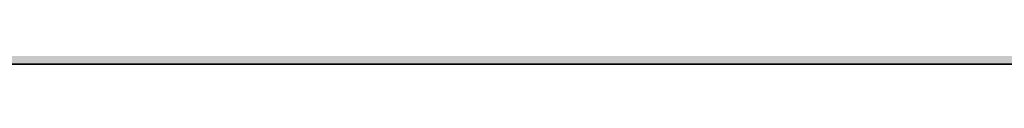
# Model space of a CAD drawing. Units: inches. Extents: x 2091 to 2899, y 967 to 2217.
# Tile 29 of 256: x 2351 to 2390, y 1091 to 1091. Entities that reach past the tile are written whole.
import ezdxf

# ---------------------------------------------------------------- set-up
doc = ezdxf.new("R2010")
doc.units = ezdxf.units.IN
doc.layers.add('A-WALL-PATT', color=141, linetype='Continuous', lineweight=13, true_color=0xadddf7)
doc.layers.add('C-PROP', color=7, linetype='Continuous', lineweight=35)

msp = doc.modelspace()

# ---------------------------------------------------------------- hatches: boundary and pattern name
at = {"layer": 'A-WALL-PATT'}
h = msp.add_hatch(color=256, dxfattribs=at)
h.dxf.hatch_style = 1
h.paths.add_polyline_path([(2212.144, 1941.419), (2387.644, 1941.419), (2387.644, 1824.419), (2392.144, 1824.419), (2392.144, 1941.419), (2609.644, 1941.419), (2609.644, 1825.919), (2614.144, 1825.919), (2614.144, 1941.419), (2794.144, 1941.419), (2794.144, 1928.762), (2803.144, 1928.762), (2803.144, 2050.919), (2203.144, 2050.919), (2203.144, 1900.758), (2212.144, 1900.758)])
h.paths.add_polyline_path([(2212.144, 1945.919), (2212.144, 2041.919), (2794.144, 2041.919), (2794.144, 1945.919), (2402.248, 1945.919), (2401.102, 1945.776), (2398.702, 1945.776)], flags=16)
h.paths.add_polyline_path([(2230.23, 1948.063), (2227.35, 1949.503), (2225.91, 1951.903), (2223.99, 1952.863), (2223.03, 1955.263), (2222.07, 1959.583), (2222.07, 1963.423), (2223.03, 1965.663), (2223.99, 1965.343), (2225.586, 1963.861), (2226.912, 1964.957), (2226.949, 1965.939), (2227.778, 1966.952), (2228.2, 1968.879), (2230.71, 1964.863), (2233.59, 1966.303), (2233.607, 1966.332), (2233.773, 1964.938), (2234.634, 1963.676), (2235.03, 1963.903), (2236.282, 1965.572), (2235.99, 1962.943), (2237.955, 1957.54), (2238.39, 1957.903), (2239.216, 1960.306), (2238.655, 1966.385), (2238.693, 1966.438), (2238.841, 1967.5), (2238.78, 1967.687), (2238.881, 1967.787), (2238.667, 1966.252), (2239.216, 1960.306), (2238.39, 1957.903), (2236.95, 1956.703), (2234.55, 1949.983)], flags=0)
h.paths.add_polyline_path([(2278.012, 1948.063), (2276.496, 1947.873), (2275.85, 1947.689), (2274.652, 1947.103)], flags=0)
h.paths.add_polyline_path([(2269.852, 1955.743), (2268.276, 1956.629), (2270.867, 1956.348), (2269.372, 1958.143), (2268.715, 1959.192), (2270.57, 1958.729), (2268.581, 1961.906), (2270.812, 1960.892), (2270.812, 1963.423), (2271.393, 1964.779), (2270.292, 1966.156), (2271.772, 1965.663), (2272.141, 1966.525), (2273.93, 1965.929), (2275.63, 1968.054), (2276.332, 1966.722), (2276.52, 1966.952), (2276.942, 1968.879), (2277.734, 1967.611), (2278.14, 1969.465), (2279.659, 1967.034), (2280.412, 1966.783), (2280.949, 1967.589), (2281.61, 1967.369), (2282.133, 1968.154), (2282.349, 1966.333), (2282.35, 1966.333), (2283.408, 1968.095), (2283.713, 1965.524), (2284.32, 1964.634), (2284.512, 1964.889), (2284.235, 1965.705), (2284.5, 1967.319), (2284.908, 1965.417), (2285.396, 1966.069), (2285.433, 1966.291), (2285.473, 1966.171), (2286.354, 1967.345), (2286.222, 1966.158), (2287.663, 1968.08), (2287.714, 1968.443), (2288.482, 1969.017), (2288.574, 1968.729), (2288.917, 1969.069), (2288.607, 1966.838), (2288.929, 1963.351), (2288.935, 1963.357), (2288.93, 1963.34), (2289.015, 1962.414), (2290.111, 1963.875), (2290.133, 1963.943), (2290.218, 1964.017), (2290.111, 1963.875), (2289.156, 1960.892), (2288.594, 1959.257), (2288.572, 1959.103), (2289.532, 1960.543), (2290.012, 1962.463), (2290.192, 1962.643), (2289.77, 1959.689), (2286.89, 1957.289), (2284.49, 1950.569), (2283.315, 1950.046), (2283.292, 1949.983), (2280.29, 1948.649), (2281.13, 1948.649), (2282.57, 1948.169), (2283.205, 1948.063), (2278.972, 1948.063), (2276.092, 1949.503), (2274.652, 1951.903), (2272.732, 1952.863)], flags=0)
h.paths.add_polyline_path([(2271.159, 1958.022), (2272.97, 1955.849), (2272.01, 1960.169), (2272.01, 1964.009), (2272.624, 1965.443), (2274.328, 1963.861), (2275.654, 1964.957), (2275.638, 1964.539), (2277.412, 1966.007), (2277.033, 1965.157), (2276.83, 1964.976), (2276.766, 1963.295), (2277.45, 1962.66), (2279.452, 1964.863), (2282.332, 1966.303), (2283.53, 1966.889), (2283.295, 1966.771), (2283.913, 1963.885), (2284.899, 1964.448), (2284.732, 1962.943), (2286.697, 1957.54), (2287.132, 1957.903), (2287.542, 1959.095), (2287.779, 1958.442), (2285.683, 1956.695), (2285.877, 1959.795), (2284.732, 1962.943), (2284.899, 1964.448), (2283.913, 1963.885), (2284.224, 1962.434), (2283.424, 1963.605), (2281.61, 1962.569), (2281.13, 1960.169), (2282.09, 1956.329), (2283.05, 1952.969), (2282.57, 1950.569), (2280.17, 1948.649), (2279.883, 1948.792), (2278.972, 1948.063), (2278.972, 1949.023), (2278.672, 1949.397), (2277.29, 1950.089), (2275.85, 1952.489), (2273.93, 1953.449), (2272.49, 1954.889), (2271.922, 1954.889), (2271.772, 1955.263)], flags=0)
h.paths.add_polyline_path([(2311.994, 1955.743), (2312.063, 1955.674), (2312.055, 1955.709)], flags=0)
h.paths.add_polyline_path([(2331.956, 1963.952), (2333.396, 1965.392), (2331.077, 1963.357), (2330.999, 1963.112)], flags=0)
h.paths.add_polyline_path([(2310.554, 1954.303), (2307.04, 1956.28), (2310.763, 1955.876), (2312.474, 1953.823), (2313.434, 1951.423), (2315.354, 1950.463), (2316.794, 1948.063), (2317.466, 1947.727), (2319.369, 1947.965), (2317.754, 1949.983), (2317.57, 1950.61), (2316.794, 1951.903), (2314.874, 1952.863), (2313.914, 1955.263), (2311.514, 1958.143), (2309.375, 1961.559), (2311.514, 1960.337), (2311.514, 1961.983), (2310.605, 1963.12), (2311.727, 1962.479), (2312.418, 1964.093), (2312.256, 1964.296), (2313.194, 1963.983), (2313.914, 1965.663), (2314.647, 1965.419), (2315.354, 1966.303), (2316.794, 1967.743), (2316.157, 1966.947), (2317.034, 1965.282), (2317.223, 1965.512), (2317.777, 1968.046), (2318.474, 1966.722), (2318.663, 1966.952), (2319.084, 1968.879), (2321.207, 1965.482), (2322.161, 1966.914), (2322.554, 1966.783), (2322.786, 1967.131), (2322.882, 1966.324), (2323.312, 1965.722), (2323.651, 1965.891), (2324.396, 1967.133), (2324.657, 1964.938), (2324.972, 1964.477), (2325.387, 1967.001), (2325.941, 1964.418), (2327.229, 1966.136), (2327.166, 1965.572), (2328.059, 1966.763), (2328.225, 1966.247), (2329.668, 1967.677), (2329.665, 1967.687), (2329.765, 1967.787), (2329.551, 1966.252), (2330.1, 1960.306), (2329.333, 1958.073), (2329.313, 1957.935), (2329.634, 1958.203), (2330.234, 1959.103), (2330.714, 1961.023), (2331.034, 1961.343), (2330.714, 1959.103), (2329.634, 1958.203), (2329.274, 1957.663), (2327.712, 1956.361), (2325.434, 1949.983), (2324.334, 1949.494), (2323.994, 1948.543), (2319.674, 1946.623), (2316.794, 1948.063), (2315.354, 1950.463), (2313.434, 1951.423)], flags=0)
h.paths.add_polyline_path([(2321.336, 1947.952), (2321.114, 1948.063), (2321.114, 1949.023), (2319.194, 1951.423), (2316.794, 1959.583), (2316.663, 1959.583), (2315.354, 1958.143), (2314.394, 1958.143), (2313.148, 1958.709), (2312.954, 1959.583), (2312.954, 1960.892), (2315.834, 1959.583), (2316.663, 1959.583), (2317.315, 1960.299), (2315.03, 1962.421), (2316.356, 1963.517), (2316.372, 1963.952), (2316.47, 1963.861), (2317.796, 1964.957), (2317.755, 1963.89), (2319.175, 1965.157), (2319.498, 1965.881), (2321.114, 1965.343), (2323.236, 1962.372), (2325.686, 1963.773), (2325.543, 1962.481), (2325.199, 1963.494), (2324.479, 1963.082), (2324.926, 1960.994), (2324.078, 1962.236), (2322.415, 1961.286), (2322.074, 1959.583), (2323.034, 1955.743), (2323.994, 1952.383), (2323.514, 1949.983), (2322.143, 1948.886), (2322.074, 1948.543)], flags=0)
h.paths.add_polyline_path([(2320.207, 1963.337), (2320.154, 1963.423), (2320.394, 1963.543)], flags=0)
h.paths.add_polyline_path([(2353.851, 1965.811), (2354.031, 1965.751), (2354.331, 1966.451), (2354.331, 1966.931)], flags=0)
h.paths.add_polyline_path([(2359.021, 1969.026), (2359.098, 1968.902), (2359.234, 1969.52), (2359.234, 1970)], flags=0)
h.paths.add_polyline_path([(2358.257, 1966.682), (2357.984, 1966.348), (2358.211, 1966.146), (2358.41, 1966.39)], flags=0)
h.paths.add_polyline_path([(2357.768, 1966.059), (2357.732, 1965.105), (2357.751, 1965.121), (2357.77, 1965.607), (2357.77, 1966.058)], flags=0)
h.paths.add_polyline_path([(2359.112, 1965.305), (2359.112, 1964.825), (2359.845, 1966.468), (2359.845, 1966.948)], flags=0)
h.paths.add_polyline_path([(2360.224, 1966.621), (2360.699, 1969.363), (2360.699, 1969.843), (2360.211, 1967.026), (2360.211, 1966.643)], flags=0)
h.paths.add_polyline_path([(2363.451, 1967.891), (2363.451, 1968.371), (2362.491, 1966.931), (2362.656, 1966.699)], flags=0)
h.paths.add_polyline_path([(2364.476, 1966.079), (2365.851, 1968.371), (2365.851, 1968.851), (2364.428, 1966.48)], flags=0)
h.paths.add_polyline_path([(2366.314, 1965.853), (2366.367, 1965.696), (2366.803, 1968.346), (2366.803, 1968.826)], flags=0)
h.paths.add_polyline_path([(2367.165, 1965.804), (2367.291, 1966.931), (2367.291, 1967.411), (2367.103, 1965.72)], flags=0)
h.paths.add_polyline_path([(2370.037, 1959.974), (2371.014, 1963.025), (2371.014, 1963.505), (2370.037, 1960.454)], flags=0)
h.paths.add_polyline_path([(2371.611, 1960.211), (2372.571, 1961.651), (2372.571, 1962.131), (2371.803, 1960.979)], flags=0)
h.paths.add_polyline_path([(2350.874, 1956.005), (2351.931, 1955.891), (2354.491, 1953.331), (2353.851, 1954.931), (2351.451, 1957.811), (2347.936, 1963.426), (2347.936, 1963.906), (2351.451, 1958.291), (2353.705, 1955.585), (2352.891, 1959.251), (2352.891, 1959.731), (2352.891, 1961.925), (2356.731, 1959.731), (2358.454, 1961.627), (2354.811, 1965.011), (2355.031, 1965.286), (2358.691, 1961.887), (2361.531, 1965.011), (2364.376, 1966.433), (2364.524, 1965.187), (2365.454, 1963.824), (2365.881, 1964.068), (2365.371, 1966.451), (2365.371, 1966.931), (2366.811, 1960.211), (2366.811, 1959.731), (2366.389, 1952.981), (2367.771, 1956.851), (2368.641, 1957.576), (2366.811, 1962.611), (2366.811, 1963.091), (2368.775, 1957.688), (2369.211, 1958.051), (2370.002, 1960.352), (2369.475, 1966.053), (2369.513, 1966.106), (2369.514, 1966.111), (2369.475, 1966.533), (2369.513, 1966.586), (2369.615, 1967.313), (2369.183, 1968.659), (2369.183, 1969.139), (2369.601, 1967.835), (2369.701, 1967.934), (2369.718, 1968.055), (2370.145, 1968.374), (2369.779, 1968.011), (2369.701, 1967.454), (2370.468, 1968.214), (2369.675, 1967.266), (2369.514, 1966.111), (2370.037, 1960.454), (2370.037, 1959.974), (2369.442, 1958.243), (2370.651, 1959.251), (2371.046, 1962.018), (2371.131, 1962.131), (2370.651, 1958.771), (2367.771, 1956.371), (2365.371, 1949.651), (2362.079, 1948.188), (2363.451, 1947.731), (2361.051, 1947.731), (2360.091, 1947.731), (2357.104, 1947.357), (2360.091, 1948.211), (2358.171, 1949.171), (2356.731, 1951.571), (2354.811, 1952.531), (2351.931, 1955.411)], flags=0)
h.paths.add_polyline_path([(2361.051, 1948.691), (2359.131, 1951.091), (2356.731, 1959.251), (2355.771, 1959.251), (2352.891, 1960.56), (2352.891, 1961.445), (2355.891, 1959.731), (2356.731, 1959.731), (2356.837, 1959.368), (2361.531, 1964.531), (2363.248, 1965.389), (2364.925, 1963.042), (2362.491, 1961.651), (2362.064, 1959.517), (2362.971, 1955.891), (2363.931, 1952.531), (2363.931, 1952.051), (2363.451, 1949.651), (2361.051, 1947.731)], flags=0)
h.paths.add_polyline_path([(2359.131, 1951.571), (2359.291, 1951.371), (2361.051, 1954.451), (2361.051, 1954.931)], flags=0)
h.paths.add_polyline_path([(2357.22, 1966.546), (2356.793, 1968.815), (2356.793, 1969.295), (2357.22, 1967.026)], flags=0)
h.paths.add_polyline_path([(2361.051, 1954.451), (2361.531, 1958.771), (2361.531, 1959.251), (2361.051, 1954.931)], flags=0)
h.paths.add_polyline_path([(2402.548, 1948.486), (2402.302, 1948.416), (2402.59, 1948.416)], flags=0)
h.paths.add_polyline_path([(2394.142, 1956.096), (2395.685, 1954.553), (2396.72, 1953.971), (2396.062, 1955.616), (2395.241, 1956.601), (2395.879, 1956.442), (2395.102, 1959.936), (2395.102, 1963.776), (2396.062, 1966.016), (2397.022, 1965.696), (2398.618, 1964.214), (2399.944, 1965.31), (2399.981, 1966.292), (2400.811, 1967.305), (2401.232, 1969.232), (2403.538, 1965.543), (2403.942, 1967.389), (2404.702, 1967.136), (2405.46, 1966.075), (2406.622, 1966.656), (2406.64, 1966.685), (2406.805, 1965.291), (2406.926, 1965.115), (2407.342, 1964.976), (2407.874, 1965.774), (2408.169, 1964.398), (2409.315, 1965.925), (2409.217, 1965.051), (2409.445, 1963.131), (2410.306, 1961.87), (2410.702, 1962.096), (2411.442, 1963.082), (2411.165, 1963.898), (2411.616, 1966.64), (2411.725, 1966.791), (2411.873, 1967.853), (2411.813, 1968.041), (2411.913, 1968.14), (2411.699, 1966.605), (2412.248, 1960.659), (2413.225, 1963.71), (2414.378, 1964.721), (2414.513, 1965.693), (2414.453, 1965.881), (2414.553, 1965.98), (2414.378, 1964.721), (2414.52, 1964.846), (2414.365, 1964.631), (2414.339, 1964.445), (2414.888, 1958.499), (2414.062, 1956.096), (2412.622, 1954.896), (2410.171, 1948.033), (2410.017, 1948.084), (2405.902, 1946.256), (2405.902, 1947.216), (2405.204, 1948.089), (2404.222, 1948.416), (2403.262, 1948.416), (2400.382, 1949.856), (2399.662, 1951.056), (2397.982, 1952.736), (2397.022, 1953.216), (2395.685, 1954.553), (2392.657, 1956.257)], flags=0)
h.paths.add_polyline_path([(2409.086, 1964.407), (2409.13, 1964.276), (2409.262, 1964.496)], flags=0)
h.paths.add_polyline_path([(2397.742, 1961.616), (2398.702, 1963.856), (2399.662, 1963.536), (2401.427, 1965.741), (2401.791, 1966.559), (2402.071, 1965.071), (2402.836, 1964.393), (2403.262, 1964.915), (2403.338, 1964.771), (2402.616, 1963.976), (2402.499, 1960.902), (2403.543, 1959.932), (2404.413, 1960.89), (2404.702, 1962.336), (2407.916, 1964.172), (2409.52, 1961.927), (2410.987, 1957.893), (2411.422, 1958.256), (2412.048, 1960.076), (2412.41, 1959.079), (2411.676, 1958.467), (2411.662, 1958.256), (2411.626, 1958.426), (2409.982, 1957.056), (2407.582, 1950.336), (2403.262, 1948.416), (2403.262, 1949.376), (2401.342, 1951.776), (2399.417, 1958.324), (2397.742, 1959.085), (2397.742, 1959.97), (2397.102, 1960.336), (2397.742, 1960.045)], flags=0)
h.paths.add_polyline_path([(2405.902, 1952.976), (2405.95, 1953.408), (2406.017, 1953.176)], flags=0)
h.paths.add_polyline_path([(2449.818, 1967.114), (2449.752, 1967.136), (2449.794, 1967.078)], flags=0)
h.paths.add_polyline_path([(2451.698, 1966.618), (2451.741, 1966.69), (2451.692, 1966.666)], flags=0)
h.paths.add_polyline_path([(2454.344, 1965.738), (2455.752, 1967.616), (2455.992, 1968.096), (2454.364, 1965.925)], flags=0)
h.paths.add_polyline_path([(2457.547, 1968.864), (2457.787, 1969.344), (2457.054, 1968.796), (2457.008, 1968.46)], flags=0)
h.paths.add_polyline_path([(2456.922, 1967.857), (2456.802, 1968.229), (2456.723, 1967.66)], flags=0)
h.paths.add_polyline_path([(2457.302, 1967.377), (2457.542, 1967.857), (2456.81, 1966.84), (2456.741, 1966.7), (2456.749, 1966.608)], flags=0)
h.paths.add_polyline_path([(2458.275, 1963.71), (2458.155, 1963.335), (2460.354, 1965.265), (2460.594, 1965.745)], flags=0)
h.paths.add_polyline_path([(2458.392, 1962.816), (2458.364, 1962.618), (2459.592, 1964.256), (2459.832, 1964.736)], flags=0)
h.paths.add_polyline_path([(2459.352, 1962.816), (2459.272, 1962.496), (2460.072, 1963.296), (2460.312, 1963.776)], flags=0)
h.paths.add_polyline_path([(2458.68, 1960.608), (2458.632, 1960.416), (2459.592, 1961.856), (2459.832, 1962.336)], flags=0)
h.paths.add_polyline_path([(2437.838, 1956.243), (2439.192, 1956.096), (2441.352, 1953.936), (2440.872, 1955.136), (2438.472, 1958.016), (2438.072, 1958.656), (2438.712, 1958.496), (2440.64, 1956.183), (2439.912, 1959.456), (2439.912, 1963.296), (2441.352, 1966.656), (2441.592, 1967.136), (2441.112, 1966.016), (2442.072, 1965.696), (2443.989, 1968.092), (2444.241, 1966.751), (2444.917, 1966.152), (2445.677, 1967.08), (2446.255, 1969.725), (2446.495, 1970.205), (2446.282, 1969.232), (2447.363, 1967.503), (2447.72, 1969.568), (2447.96, 1970.048), (2447.485, 1967.307), (2448.792, 1965.216), (2448.472, 1964.864), (2448.552, 1964.736), (2451.452, 1966.186), (2451.615, 1964.811), (2452.308, 1963.796), (2453.235, 1964.326), (2454.072, 1960.416), (2453.629, 1953.318), (2454.792, 1956.576), (2455.032, 1957.056), (2455.719, 1957.628), (2453.832, 1962.816), (2453.941, 1963.794), (2453.335, 1965.578), (2453.824, 1968.551), (2454.064, 1969.031), (2453.575, 1966.058), (2454.04, 1964.688), (2453.832, 1962.816), (2455.719, 1957.628), (2456.367, 1958.168), (2457.058, 1960.179), (2457.298, 1960.659), (2456.472, 1958.256), (2457.718, 1959.294), (2457.672, 1958.976), (2454.89, 1956.657), (2453.614, 1953.085), (2453.592, 1952.736), (2453.352, 1952.256), (2453.36, 1952.372), (2452.632, 1950.336), (2452.392, 1949.856), (2449.204, 1948.439), (2450.712, 1947.936), (2448.072, 1947.936), (2447.112, 1947.936), (2444.552, 1947.616), (2447.2, 1948.372), (2445.192, 1949.376), (2443.752, 1951.776), (2441.832, 1952.736), (2438.952, 1955.616)], flags=0)
h.paths.add_polyline_path([(2443.992, 1959.936), (2444.04, 1959.773), (2444.122, 1959.862)], flags=0)
h.paths.add_polyline_path([(2442.912, 1959.936), (2443.032, 1959.936), (2442.446, 1960.202)], flags=0)
h.paths.add_polyline_path([(2444.983, 1965.02), (2445.279, 1965.265), (2445.519, 1965.745), (2444.994, 1965.31)], flags=0)
h.paths.add_polyline_path([(2446.133, 1965.03), (2446.33, 1965.471), (2444.97, 1964.258), (2444.73, 1963.778)], flags=0)
h.paths.add_polyline_path([(2442.792, 1959.456), (2443.752, 1959.456), (2446.152, 1951.296), (2446.412, 1951.751), (2446.392, 1951.776), (2448.081, 1954.73), (2448.552, 1958.976), (2441.832, 1965.216), (2442.155, 1965.619), (2448.792, 1959.456), (2448.312, 1955.136), (2448.072, 1954.656), (2446.412, 1951.751), (2448.312, 1949.376), (2448.312, 1948.416), (2450.541, 1950.199), (2450.952, 1952.256), (2449.992, 1955.616), (2449.032, 1959.456), (2449.512, 1961.856), (2449.752, 1962.336), (2449.675, 1961.949), (2452.995, 1963.846), (2453.064, 1963.519), (2452.885, 1963.783), (2449.675, 1961.949), (2449.272, 1959.936), (2450.232, 1956.096), (2451.192, 1952.736), (2450.712, 1950.336), (2450.472, 1949.856), (2448.072, 1947.936), (2448.072, 1948.536), (2445.432, 1949.856), (2443.992, 1952.256), (2442.072, 1953.216), (2441.112, 1955.616), (2440.152, 1959.936), (2440.152, 1960.656)], flags=0)
h.paths.add_polyline_path([(2456.692, 1966.986), (2457.608, 1968.081), (2457.848, 1968.561), (2456.932, 1967.466)], flags=0)
h.paths.add_polyline_path([(2489.897, 1966.58), (2489.943, 1966.189), (2490.747, 1967.53), (2491.319, 1968.951)], flags=0)
h.paths.add_polyline_path([(2473.562, 1956.407), (2477.14, 1956.019), (2476.955, 1956.241), (2475.108, 1957.28), (2476.347, 1956.97), (2475.187, 1958.824), (2476.919, 1958.391), (2475.412, 1960.799), (2477.787, 1959.719), (2477.787, 1962.25), (2477.637, 1962.438), (2477.823, 1962.332), (2478.359, 1963.584), (2478.359, 1963.671), (2477.324, 1964.965), (2478.715, 1964.501), (2479.319, 1965.911), (2480.279, 1965.591), (2481.784, 1967.472), (2482.116, 1965.705), (2482.881, 1965.028), (2483.209, 1965.429), (2483.22, 1965.715), (2483.076, 1965.989), (2483.712, 1966.766), (2484.13, 1968.679), (2484.702, 1970.1), (2484.489, 1969.127), (2486.503, 1965.905), (2487.387, 1965.61), (2488.153, 1966.759), (2488.717, 1965.97), (2489.2, 1966.212), (2489.331, 1965.111), (2490.394, 1963.622), (2490.661, 1963.775), (2490.494, 1964.554), (2490.923, 1963.925), (2491.319, 1964.151), (2491.333, 1964.17), (2491.21, 1964.532), (2491.282, 1964.966), (2491.426, 1964.293), (2494.076, 1967.828), (2494.498, 1966.515), (2494.598, 1966.614), (2494.689, 1967.27), (2495.107, 1967.582), (2495.13, 1967.748), (2495.07, 1967.936), (2495.17, 1968.035), (2495.032, 1967.044), (2495.754, 1967.759), (2494.982, 1966.686), (2494.956, 1966.5), (2495.479, 1960.837), (2495.91, 1962.184), (2496.482, 1963.605), (2496.073, 1962.327), (2496.769, 1962.938), (2496.599, 1962.711), (2496.119, 1959.351), (2496.733, 1960.272), (2496.987, 1961.29), (2497.559, 1962.711), (2497.079, 1960.791), (2496.507, 1959.37), (2495.547, 1957.93), (2492.759, 1955.606), (2490.839, 1950.231), (2490.267, 1948.81), (2485.947, 1946.89), (2483.067, 1948.33), (2481.627, 1950.73), (2479.707, 1951.69), (2476.827, 1954.57)], flags=0)
h.paths.add_polyline_path([(2485.577, 1948.313), (2485.559, 1948.311), (2485.579, 1948.311)], flags=0)
h.paths.add_polyline_path([(2478.645, 1954.551), (2478.109, 1956.963), (2479.319, 1955.511), (2480.279, 1953.111), (2482.199, 1952.151), (2483.639, 1949.751), (2486.519, 1948.311), (2486.519, 1949.271), (2484.739, 1951.496), (2484.027, 1950.25), (2481.627, 1958.41), (2482.375, 1959.233), (2482.199, 1959.831), (2483.198, 1960.929), (2479.707, 1964.17), (2480.603, 1965.29), (2481.875, 1964.109), (2482.666, 1964.764), (2482.615, 1963.422), (2482.989, 1963.075), (2484.008, 1963.984), (2484.684, 1965.498), (2484.58, 1965.405), (2485.357, 1967.147), (2485.121, 1965.781), (2486.427, 1963.69), (2488.145, 1964.549), (2489.822, 1962.202), (2490.747, 1962.73), (2492, 1964.4), (2492.076, 1965.087), (2492.213, 1964.684), (2492.485, 1965.047), (2492.279, 1963.191), (2494.244, 1957.788), (2494.563, 1958.054), (2494.933, 1959.133), (2495.505, 1960.554), (2494.679, 1958.151), (2494.107, 1956.73), (2494.563, 1958.054), (2493.409, 1957.092), (2491.707, 1961.77), (2492, 1964.4), (2490.747, 1962.73), (2487.712, 1960.996), (2487.479, 1959.831), (2488.439, 1955.991), (2489.399, 1952.631), (2488.919, 1950.231), (2488.577, 1949.957), (2488.347, 1948.81), (2487.652, 1948.254), (2487.479, 1948.311), (2486.519, 1948.311), (2483.639, 1949.751), (2482.199, 1952.151), (2480.279, 1953.111), (2478.839, 1954.551)], flags=0)
h.paths.add_polyline_path([(2526.648, 1966.988), (2526.517, 1967.031), (2526.6, 1966.915)], flags=0)
h.paths.add_polyline_path([(2528.471, 1966.447), (2528.574, 1966.62), (2528.457, 1966.561)], flags=0)
h.paths.add_polyline_path([(2534.133, 1967.496), (2534.157, 1967.543), (2534.06, 1967.408)], flags=0)
h.paths.add_polyline_path([(2536.162, 1964.051), (2535.157, 1962.711), (2535.101, 1962.316), (2536.117, 1963.671), (2536.421, 1964.278)], flags=0)
h.paths.add_polyline_path([(2535.157, 1959.831), (2536.117, 1961.271), (2536.597, 1962.231), (2535.253, 1960.215)], flags=0)
h.paths.add_polyline_path([(2513.249, 1956.285), (2516.221, 1955.963), (2514.997, 1957.431), (2514.196, 1958.712), (2515.477, 1958.391), (2516.932, 1956.646), (2516.437, 1958.871), (2516.437, 1962.711), (2516.873, 1963.727), (2515.346, 1965.635), (2517.397, 1964.951), (2517.877, 1966.071), (2518.357, 1967.031), (2517.877, 1965.911), (2518.837, 1965.591), (2520.487, 1967.653), (2520.766, 1966.166), (2521.53, 1965.489), (2521.781, 1965.795), (2521.801, 1966.307), (2521.478, 1966.921), (2521.246, 1967.126), (2521.178, 1967.491), (2521.478, 1966.921), (2522.01, 1966.449), (2522.257, 1966.75), (2522.78, 1969.14), (2523.26, 1970.1), (2523.047, 1969.127), (2524.673, 1966.526), (2526.037, 1966.071), (2526.795, 1965.01), (2527.977, 1965.601), (2528.14, 1964.227), (2528.665, 1963.458), (2529.389, 1963.872), (2529.33, 1964.147), (2529.481, 1963.925), (2529.877, 1964.151), (2529.984, 1964.293), (2529.789, 1965.203), (2530.062, 1964.398), (2532.802, 1968.051), (2533.148, 1966.976), (2533.248, 1967.075), (2533.339, 1967.731), (2533.673, 1967.98), (2533.728, 1968.035), (2533.514, 1966.5), (2534.025, 1960.972), (2534.56, 1962.645), (2535.04, 1963.605), (2534.063, 1960.554), (2533.237, 1958.151), (2534.288, 1959.027), (2534.197, 1958.391), (2531.513, 1956.154), (2529.397, 1950.231), (2528.917, 1949.271), (2526.449, 1948.174), (2527.477, 1947.831), (2530.357, 1947.351), (2524.597, 1947.351), (2521.717, 1948.791), (2520.277, 1951.191), (2518.357, 1952.151), (2515.477, 1955.031)], flags=0)
h.paths.add_polyline_path([(2523.935, 1967.19), (2523.62, 1966.484), (2523.77, 1966.242)], flags=0)
h.paths.add_polyline_path([(2518.837, 1953.111), (2517.877, 1955.511), (2516.885, 1959.977), (2516.917, 1959.962), (2516.917, 1962.025), (2520.757, 1959.831), (2522.025, 1961.226), (2518.357, 1964.631), (2519.003, 1965.438), (2520.433, 1964.109), (2521.301, 1964.827), (2521.245, 1963.355), (2525.638, 1959.276), (2526.037, 1961.271), (2529.397, 1963.191), (2530.65, 1964.861), (2530.665, 1964.998), (2530.692, 1964.917), (2531.088, 1965.445), (2530.946, 1964.169), (2530.692, 1964.917), (2529.397, 1963.191), (2526.363, 1961.457), (2526.037, 1959.831), (2526.997, 1955.991), (2527.957, 1952.631), (2527.477, 1950.231), (2527.134, 1949.957), (2526.974, 1949.154), (2526.697, 1949.031), (2524.597, 1947.351), (2524.597, 1948.311), (2524.277, 1948.711), (2522.197, 1949.751), (2520.757, 1952.151)], flags=0)
h.paths.add_polyline_path([(2520.277, 1958.871), (2520.853, 1959.505), (2523.157, 1951.671), (2524.614, 1954.22), (2524.597, 1954.071), (2522.677, 1950.711)], flags=0)
h.paths.add_polyline_path([(2559.371, 1966.311), (2559.398, 1966.325), (2559.402, 1966.345)], flags=0)
h.paths.add_polyline_path([(2549.771, 1957.191), (2552.651, 1954.311), (2552.134, 1955.603), (2550.611, 1957.431), (2547.096, 1963.046), (2545.776, 1965.206), (2549.291, 1959.591), (2551.691, 1956.711), (2550.793, 1960.752), (2550.731, 1960.78), (2550.731, 1964.871), (2551.691, 1967.111), (2552.651, 1966.791), (2554.247, 1965.309), (2555.034, 1965.96), (2555.582, 1966.645), (2555.61, 1967.387), (2556.439, 1968.401), (2556.861, 1970.327), (2559.371, 1966.311), (2560.691, 1964.151), (2562.409, 1965.01), (2561.651, 1966.071), (2560.331, 1968.231), (2561.758, 1966.233), (2562.347, 1967.116), (2562.434, 1966.387), (2563.128, 1965.37), (2563.571, 1965.591), (2563.588, 1965.62), (2563.363, 1967.524), (2563.722, 1965.844), (2565.06, 1968.073), (2564.733, 1965.129), (2565.118, 1963.333), (2567.445, 1966.436), (2567.316, 1967.833), (2567.354, 1967.886), (2567.502, 1968.948), (2567.441, 1969.136), (2567.542, 1969.235), (2567.328, 1967.7), (2567.877, 1961.754), (2568.747, 1964.47), (2568.636, 1965.673), (2568.674, 1965.726), (2568.822, 1966.788), (2568.761, 1966.976), (2568.862, 1967.075), (2568.648, 1965.54), (2568.726, 1964.693), (2568.854, 1964.805), (2568.747, 1964.47), (2568.817, 1963.706), (2568.971, 1963.911), (2568.866, 1963.177), (2569.197, 1959.594), (2568.371, 1957.191), (2566.931, 1955.991), (2564.62, 1949.521), (2564.651, 1949.511), (2564.617, 1949.511), (2564.531, 1949.271), (2560.211, 1947.351), (2557.331, 1948.791), (2556.045, 1950.934), (2556.011, 1950.951), (2555.857, 1951.208), (2553.971, 1952.151), (2551.091, 1955.031), (2546.65, 1957.53)], flags=0)
h.paths.add_polyline_path([(2567.026, 1959.33), (2567.035, 1959.305), (2567.051, 1959.351)], flags=0)
h.paths.add_polyline_path([(2551.968, 1962.518), (2553.011, 1964.951), (2553.971, 1964.631), (2555.567, 1963.149), (2556.893, 1964.246), (2556.93, 1965.227), (2557.144, 1965.489), (2556.42, 1966.131), (2556.391, 1966.105), (2556.38, 1966.166), (2556.42, 1966.131), (2556.952, 1966.605), (2557.092, 1966.919), (2557.571, 1966.01), (2557.759, 1966.241), (2557.418, 1964.68), (2556.893, 1964.246), (2556.807, 1961.998), (2560.691, 1958.391), (2560.636, 1957.893), (2560.811, 1957.191), (2561.771, 1953.831), (2561.291, 1951.431), (2559.11, 1949.687), (2559.156, 1949.629), (2563.027, 1951.349), (2562.611, 1949.271), (2560.211, 1947.351), (2560.211, 1948.311), (2559.251, 1949.511), (2558.891, 1949.511), (2558.891, 1949.961), (2558.291, 1950.711), (2558.054, 1951.518), (2556.971, 1952.871), (2555.068, 1959.341), (2552.051, 1961.065), (2552.051, 1962.471)], flags=0)
h.paths.add_polyline_path([(2588.33, 1958.391), (2588.61, 1958.111), (2588.553, 1958.367)], flags=0)
h.paths.add_polyline_path([(2594.745, 1950.493), (2593.958, 1953.172), (2593.13, 1954.551), (2591.21, 1955.511), (2590.25, 1957.911), (2588.309, 1960.24), (2586.177, 1961.209), (2587.85, 1960.791), (2587.253, 1961.744), (2588.441, 1961.065), (2588.441, 1962.656), (2588.422, 1962.665), (2588.441, 1962.711), (2586.914, 1964.62), (2588.877, 1963.728), (2589.29, 1964.692), (2589.29, 1966.071), (2590.25, 1968.311), (2591.21, 1967.991), (2592.806, 1966.509), (2594.132, 1967.606), (2594.169, 1968.587), (2594.999, 1969.601), (2595.42, 1971.527), (2597.93, 1967.511), (2600.81, 1968.951), (2600.827, 1968.98), (2600.993, 1967.587), (2601.854, 1966.325), (2602.107, 1966.47), (2602.236, 1967.255), (2602.357, 1966.693), (2603.502, 1968.221), (2603.21, 1965.591), (2605.175, 1960.188), (2605.507, 1960.465), (2605.026, 1965.673), (2605.064, 1965.726), (2605.212, 1966.788), (2605.152, 1966.976), (2605.252, 1967.075), (2605.343, 1967.731), (2605.953, 1968.187), (2605.875, 1969.033), (2605.913, 1969.086), (2606.061, 1970.148), (2606, 1970.336), (2606.101, 1970.435), (2605.887, 1968.9), (2606.436, 1962.954), (2605.61, 1960.551), (2605.997, 1960.874), (2606.564, 1962.645), (2608.241, 1964.117), (2608.01, 1963.191), (2607.05, 1961.751), (2606.631, 1961.402), (2606.201, 1958.391), (2603.321, 1955.991), (2600.921, 1949.271), (2596.601, 1947.351), (2593.721, 1948.791), (2592.857, 1950.231), (2592.65, 1950.231)], flags=0)
h.paths.add_polyline_path([(2596.601, 1947.351), (2596.601, 1948.311), (2594.681, 1950.711), (2596.155, 1953.29), (2595.53, 1954.071), (2593.199, 1961.996), (2592.651, 1962.505), (2591.78, 1963.003), (2593.283, 1964.246), (2593.32, 1965.227), (2594.15, 1966.241), (2594.571, 1968.167), (2596.183, 1965.589), (2596.951, 1966.435), (2598.041, 1966.071), (2598.799, 1965.01), (2599.961, 1965.591), (2599.979, 1965.62), (2600.144, 1964.227), (2601.005, 1962.965), (2601.401, 1963.191), (2602.653, 1964.861), (2602.361, 1962.231), (2603.793, 1958.295), (2601.978, 1953.212), (2601.946, 1952.709), (2599.469, 1951.608), (2599.001, 1949.271)], flags=0)
h.paths.add_polyline_path([(2597.561, 1958.871), (2597.671, 1959.419), (2597.595, 1958.736)], flags=0)
h.paths.add_polyline_path([(2623.666, 1961.254), (2625.519, 1960.791), (2624.966, 1961.676), (2627.199, 1960.66), (2627.199, 1961.151), (2626.959, 1962.231), (2626.959, 1963.491), (2625.582, 1965.212), (2626.959, 1964.425), (2626.959, 1965.831), (2626.869, 1965.861), (2627.919, 1968.311), (2628.879, 1967.991), (2630.475, 1966.509), (2631.801, 1967.606), (2631.838, 1968.587), (2632.668, 1969.601), (2633.089, 1971.527), (2635.599, 1967.511), (2638.479, 1968.951), (2638.497, 1968.98), (2638.662, 1967.587), (2639.176, 1966.833), (2639.78, 1967.84), (2640.026, 1966.693), (2641.171, 1968.221), (2640.879, 1965.591), (2641.114, 1964.945), (2641.411, 1965.341), (2641.308, 1964.412), (2642.844, 1960.188), (2643.279, 1960.551), (2644.085, 1962.895), (2643.784, 1966.153), (2643.807, 1966.185), (2643.601, 1968.418), (2643.523, 1968.661), (2643.73, 1970.148), (2643.67, 1970.336), (2643.77, 1970.435), (2643.556, 1968.9), (2643.601, 1968.418), (2643.91, 1967.456), (2644.01, 1967.555), (2643.812, 1966.132), (2644.105, 1962.954), (2644.239, 1961.351), (2644.719, 1961.751), (2645.033, 1962.222), (2645.322, 1963.125), (2646.076, 1963.787), (2645.033, 1962.222), (2644.345, 1960.074), (2643.519, 1957.671), (2642.079, 1956.471), (2639.72, 1949.864), (2639.876, 1949.838), (2635.359, 1947.831), (2632.479, 1949.271), (2631.039, 1951.671), (2629.119, 1952.631), (2628.159, 1955.031), (2625.759, 1957.911)], flags=0)
h.paths.add_polyline_path([(2627.816, 1956.574), (2627.374, 1958.566), (2626.376, 1959.763), (2627.199, 1959.351), (2627.374, 1958.566), (2627.919, 1957.911), (2628.879, 1955.511), (2630.799, 1954.551), (2632.239, 1952.151), (2633.315, 1951.613), (2631.039, 1959.351), (2631.498, 1959.856), (2630.799, 1962.231), (2631.45, 1962.947), (2630.715, 1963.629), (2632.041, 1964.726), (2632.078, 1965.707), (2632.292, 1965.969), (2631.705, 1966.489), (2633.136, 1967.766), (2633.329, 1968.647), (2634.675, 1966.494), (2635.208, 1967.081), (2636.799, 1966.551), (2637.676, 1967.867), (2638.994, 1966.022), (2639.705, 1966.429), (2641.119, 1959.831), (2640.93, 1956.806), (2639.439, 1952.631), (2638.227, 1952.093), (2637.759, 1949.751), (2635.359, 1947.831), (2635.359, 1948.791), (2633.439, 1951.191), (2633.315, 1951.613), (2632.239, 1952.151), (2630.799, 1954.551), (2628.879, 1955.511)], flags=0)
h.paths.add_polyline_path([(2637.759, 1953.831), (2637.279, 1955.511), (2636.319, 1959.351), (2636.799, 1961.751), (2639.234, 1963.142), (2637.557, 1965.49), (2638.739, 1966.081), (2638.902, 1964.707), (2639.763, 1963.445), (2636.799, 1961.751), (2636.532, 1960.418), (2637.039, 1958.391), (2637.999, 1955.031)], flags=0)
h.paths.add_polyline_path([(2668.567, 1951.431), (2667.607, 1953.831), (2665.207, 1956.711), (2662.294, 1961.365), (2665.447, 1959.591), (2666.647, 1958.391), (2666.647, 1959.975), (2666.058, 1960.682), (2666.647, 1960.345), (2666.647, 1961.991), (2666.7, 1962.114), (2666.407, 1963.431), (2666.407, 1967.271), (2667.367, 1969.511), (2668.327, 1969.191), (2669.923, 1967.709), (2671.249, 1968.806), (2671.286, 1969.787), (2672.116, 1970.801), (2672.537, 1972.727), (2675.047, 1968.711), (2677.927, 1970.151), (2677.945, 1970.18), (2678.11, 1968.787), (2678.971, 1967.525), (2679.367, 1967.751), (2680.62, 1969.421), (2680.327, 1966.791), (2682.292, 1961.388), (2682.727, 1961.751), (2683.358, 1963.587), (2683.232, 1964.953), (2683.27, 1965.006), (2683.393, 1965.889), (2683.36, 1966.249), (2683.358, 1966.256), (2683.359, 1966.257), (2682.992, 1970.233), (2683.03, 1970.286), (2683.178, 1971.348), (2683.118, 1971.536), (2683.218, 1971.635), (2683.004, 1970.1), (2683.359, 1966.257), (2683.458, 1966.355), (2683.393, 1965.889), (2683.414, 1965.665), (2684.424, 1966.872), (2683.553, 1964.154), (2683.358, 1963.587), (2683.793, 1958.874), (2682.967, 1956.471), (2681.527, 1955.271), (2680.109, 1951.3), (2680.085, 1950.912), (2679.977, 1950.93), (2679.127, 1948.551), (2674.807, 1946.631), (2671.927, 1948.071), (2670.487, 1950.471)], flags=0)
h.paths.add_polyline_path([(2671.936, 1953.227), (2671.687, 1953.351), (2670.247, 1955.751), (2668.327, 1956.711), (2667.357, 1959.138), (2669.527, 1958.151), (2670.487, 1958.151), (2671.479, 1959.242), (2670.684, 1961.945), (2668.89, 1963.612), (2667.307, 1964.331), (2668.567, 1963.911), (2668.831, 1964.241), (2670.247, 1963.431), (2672.422, 1965.823), (2672.777, 1967.447), (2673.234, 1966.716), (2674.412, 1968.012), (2673.981, 1965.522), (2675.287, 1963.431), (2675.554, 1963.564), (2675.932, 1965.456), (2676.247, 1965.351), (2677.005, 1964.29), (2678.167, 1964.871), (2679.607, 1967.271), (2680.327, 1963.911), (2680.307, 1963.577), (2680.347, 1963.458), (2680.86, 1964.141), (2680.567, 1961.511), (2681.104, 1960.037), (2678.887, 1953.831), (2677.092, 1953.033), (2677.687, 1950.951), (2677.207, 1948.551), (2674.807, 1946.631), (2674.807, 1947.591), (2672.887, 1949.991)], flags=0)
h.paths.add_polyline_path([(2673.985, 1951.911), (2674.567, 1952.931), (2674.567, 1951.911), (2676.967, 1953.831), (2677.447, 1956.231), (2676.487, 1959.591), (2676.247, 1960.551), (2679.73, 1962.541), (2680.059, 1961.002), (2679.211, 1962.245), (2676.247, 1960.551), (2676.487, 1959.591), (2677.447, 1956.231), (2676.967, 1953.831), (2674.567, 1951.911)], flags=0)
h.paths.add_polyline_path([(2707.479, 1952.815), (2706.519, 1955.215), (2705.559, 1959.535), (2705.559, 1963.375), (2706.519, 1965.615), (2707.479, 1965.295), (2709.075, 1963.813), (2710.401, 1964.909), (2710.438, 1965.891), (2711.268, 1966.904), (2711.689, 1968.831), (2714.199, 1964.815), (2717.079, 1966.255), (2717.097, 1966.284), (2717.262, 1964.89), (2718.123, 1963.628), (2718.519, 1963.855), (2719.771, 1965.524), (2719.479, 1962.895), (2721.444, 1957.492), (2721.879, 1957.855), (2722.705, 1960.258), (2722.144, 1966.337), (2722.182, 1966.39), (2722.33, 1967.452), (2722.27, 1967.639), (2722.37, 1967.739), (2722.156, 1966.204), (2722.705, 1960.258), (2721.879, 1957.855), (2720.439, 1956.655), (2718.039, 1949.935), (2713.719, 1948.015), (2710.839, 1949.455), (2709.399, 1951.855)], flags=0)
h.paths.add_polyline_path([(2749.301, 1952.815), (2748.341, 1955.215), (2747.381, 1959.535), (2747.381, 1963.375), (2748.341, 1965.615), (2749.301, 1965.295), (2750.897, 1963.813), (2752.223, 1964.909), (2752.26, 1965.891), (2753.09, 1966.904), (2753.511, 1968.831), (2756.021, 1964.815), (2758.901, 1966.255), (2758.919, 1966.284), (2759.084, 1964.89), (2759.945, 1963.628), (2760.341, 1963.855), (2761.593, 1965.524), (2761.301, 1962.895), (2763.266, 1957.492), (2763.701, 1957.855), (2764.527, 1960.258), (2763.966, 1966.337), (2764.004, 1966.39), (2764.152, 1967.452), (2764.092, 1967.639), (2764.192, 1967.739), (2763.978, 1966.204), (2764.527, 1960.258), (2763.701, 1957.855), (2762.261, 1956.655), (2759.861, 1949.935), (2755.541, 1948.015), (2752.661, 1949.455), (2751.221, 1951.855)], flags=0)
h.paths.add_polyline_path([(2212.144, 1819.935), (2203.144, 1819.935), (2203.144, 1739.98), (2212.144, 1739.98), (2212.144, 1780.919), (2392.144, 1780.919), (2392.144, 1783.919), (2212.144, 1783.919)])
h.paths.add_polyline_path([(2803.144, 1847.939), (2794.144, 1847.939), (2794.144, 1785.419), (2609.644, 1785.419), (2493.876, 1785.419), (2493.876, 1780.919), (2609.644, 1780.919), (2794.144, 1780.919), (2794.144, 1696.919), (2609.376, 1696.919), (2609.376, 1742.919), (2604.876, 1742.919), (2604.876, 1644.419), (2609.376, 1644.419), (2609.376, 1692.419), (2794.144, 1692.419), (2794.144, 1668.165), (2803.144, 1668.165)])
h.paths.add_polyline_path([(2392.144, 1740.419), (2387.644, 1740.419), (2387.644, 1629.419), (2212.144, 1629.419), (2212.144, 1659.156), (2203.144, 1659.156), (2203.144, 1494.089), (2212.144, 1494.089), (2212.144, 1627.919), (2392.144, 1627.919)])
h.paths.add_polyline_path([(2457.876, 1780.919), (2453.376, 1780.919), (2453.376, 1644.419), (2568.876, 1644.419), (2568.876, 1648.919), (2457.876, 1648.919)])
h.paths.add_polyline_path([(2545.144, 1591.919), (2540.644, 1591.919), (2540.644, 1567.919), (2468.644, 1567.919), (2468.644, 1627.919), (2509.144, 1627.919), (2509.144, 1632.419), (2464.144, 1632.419), (2464.144, 1563.419), (2545.144, 1563.419)])
h.paths.add_polyline_path([(2268.644, 1555.919), (2212.144, 1555.919), (2212.144, 1551.419), (2268.644, 1551.419)], flags=17)
h.paths.add_polyline_path([(2212.144, 1413.266), (2203.144, 1413.266), (2203.144, 1233.07), (2212.144, 1233.07)])
h.paths.add_polyline_path([(2267.644, 1351.919), (2212.144, 1351.919), (2212.144, 1347.419), (2267.644, 1347.419)], flags=17)
h.paths.add_polyline_path([(2456.644, 1489.419), (2452.144, 1489.419), (2452.144, 1351.919), (2312.644, 1351.919), (2312.644, 1347.419), (2456.644, 1347.419)])
h.paths.add_polyline_path([(2472.37, 1455.419), (2467.87, 1455.419), (2467.87, 1347.419), (2472.37, 1347.419)])
h.paths.add_polyline_path([(2794.144, 1351.919), (2543.37, 1351.919), (2543.37, 1347.419), (2794.144, 1347.419)], flags=17)
h.paths.add_polyline_path([(2312.644, 1347.419), (2308.144, 1347.419), (2308.144, 1302.162), (2308.342, 1302.164), (2308.144, 1298.169), (2308.144, 1275.419), (2212.144, 1275.419), (2212.144, 1270.919), (2312.644, 1270.919)], flags=17)
h.paths.add_polyline_path([(2212.144, 1152.247), (2203.144, 1152.247), (2203.144, 1090.919), (2803.144, 1090.919), (2803.144, 1392.714), (2794.144, 1392.714), (2794.144, 1143.419), (2548.032, 1143.419), (2548.032, 1138.919), (2794.144, 1138.919), (2794.144, 1099.919), (2212.144, 1099.919)])
h.paths.add_polyline_path([(2471.532, 1266.329, 0.031658), (2467.032, 1269.946), (2467.032, 1143.419), (2471.532, 1143.419), (2471.532, 1148.819)], flags=17)
h.paths.add_polyline_path([(2803.144, 1587.341), (2794.144, 1587.341), (2794.144, 1473.537), (2803.144, 1473.537)])
h.paths.add_polyline_path([(2794.144, 1536.419), (2651.144, 1536.419), (2651.144, 1531.919), (2794.144, 1531.919)])
h.paths.add_polyline_path([(2614.144, 1620.419), (2609.644, 1620.419), (2609.644, 1536.419), (2614.144, 1536.419)])
h.paths.add_polyline_path([(2271.083, 1964.317), (2776.853, 1964.317), (2776.853, 2037.17), (2271.083, 2037.17)], flags=8)
h.paths.add_polyline_path([(2380.649, 1536.824), (2461.041, 1536.824), (2461.041, 1554.653), (2380.649, 1554.653)], flags=9)
h.paths.add_polyline_path([(2203.655, 1608.815), (2316.118, 1608.815), (2316.118, 1621.918), (2203.655, 1621.918)], flags=24)
h.paths.add_polyline_path([(2212.677, 1313.504), (2282.592, 1313.504), (2282.592, 1322.745), (2212.677, 1322.745)], flags=24)
h.paths.add_polyline_path([(2457.112, 1114.779), (2558.482, 1114.779), (2558.482, 1142.22), (2457.112, 1142.22)], flags=25)
h.paths.add_polyline_path([(2473.442, 1273.01), (2604.641, 1273.01), (2604.641, 1318.347), (2473.442, 1318.347)], flags=25)
h.paths.add_polyline_path([(2638.876, 1626.977), (2684.25, 1627.977), (2684.038, 1637.597), (2638.664, 1636.598)], flags=9)
h.paths.add_polyline_path([(2537.591, 1453.793), (2628.39, 1453.793), (2628.39, 1475.345), (2537.591, 1475.345)], flags=9)
h.paths.add_polyline_path([(2504.138, 1714.632), (2554.647, 1714.632), (2554.647, 1730.238), (2504.138, 1730.238)], flags=25)
h.paths.add_polyline_path([(2487.501, 1575.652), (2535.097, 1575.652), (2535.097, 1598.378), (2487.501, 1598.378)], flags=25)
h.paths.add_polyline_path([(2709.099, 1735.71), (2740.017, 1735.71), (2740.017, 1749.938), (2709.099, 1749.938)], flags=25)
h.paths.add_polyline_path([(2442.438, 1792.172), (2564.729, 1792.172), (2564.729, 1842), (2442.438, 1842)], flags=9)
h.paths.add_polyline_path([(2655.816, 1809.644), (2789.52, 1806.694), (2790.085, 1832.292), (2656.381, 1835.242)], flags=25)
h.paths.add_polyline_path([(2234.843, 1797.72), (2368.593, 1794.769), (2369.161, 1820.504), (2235.411, 1823.455)], flags=9)
h.paths.add_polyline_path([(2245.138, 1644.006), (2398.428, 1640.624), (2398.995, 1666.325), (2245.706, 1669.707)], flags=9)
h.paths.add_polyline_path([(2306.143, 1431.169), (2413.768, 1428.794), (2414.333, 1454.392), (2306.708, 1456.766)], flags=9)
h.paths.add_polyline_path([(2306.835, 1458.233), (2393.38, 1456.323), (2393.933, 1481.354), (2307.387, 1483.264)], flags=9)

# ---------------------------------------------------------------- linework, layer by layer
at = {"layer": 'C-PROP'}
msp.add_lwpolyline([(2203.144, 2050.919), (2803.144, 2050.919), (2803.144, 1090.919), (2203.144, 1090.919)], close=True, dxfattribs=at)

doc.saveas('drawing.dxf')
